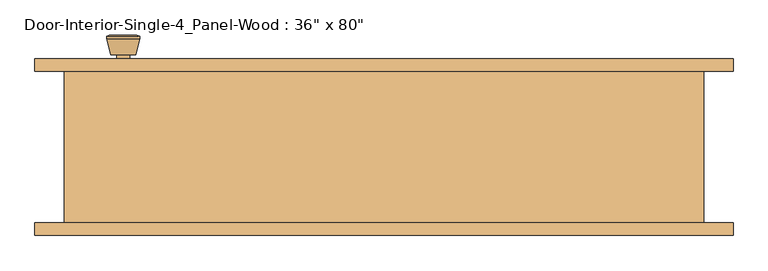
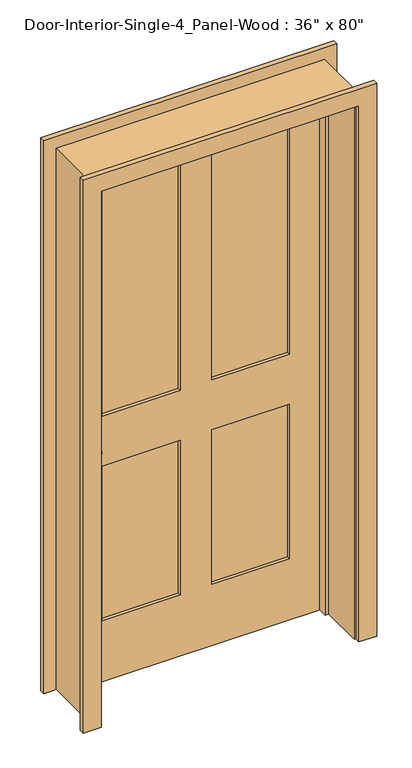
"""IFC4 building model written with IfcOpenShell, lengths in millimetres: door geometry."""

from ifc_helpers import new_model, si_unit, point, frame, frame_2d, origin, place, context, project, spatial, polyline, circle_curve, trimmed, segment, composite_curve, outline, extrude, faceted_brep, source, transform, mapped, element, save
from ifc_brep_helpers import plane_surface, cylinder_surface, revolved_surface, advanced_brep


def door_8a5afc22(model_context):
    return source(origin(), model_context, "Body", "SolidModel", [
        advanced_brep(
        [(-393.7, 70.2, 914.4), (-383.7, 70.2, 914.4), (-403.7, 70.2, 914.4), (-373.2241324, 21.2, 914.4), (-393.7, 21.2, 914.4), (-414.1758676, 21.2, 914.4), (-368.7, 23.0278681, 914.4), (-418.7, 23.0278681, 914.4), (-368.7, 26.4915463, 914.4), (-418.7, 26.4915463, 914.4), (-375.063764, 51.2, 914.4), (-412.336236, 51.2, 914.4), (-383.7, 51.2, 914.4), (-403.7, 51.2, 914.4)],
        [
            (0, 1),
            (1, 2, circle_curve(frame((-393.7, 70.2, 914.4), z_axis=(0.0, 1.0, 0.0), x_axis=(-1.0, 0.0, 0.0)), 10.0)),
            (2, 0),
            (2, 1, circle_curve(frame((-393.7, 70.2, 914.4), z_axis=(0.0, 1.0, 0.0), x_axis=(-1.0, 0.0, 0.0)), 10.0)),
            (3, 4),
            (4, 5),
            (5, 3, circle_curve(frame((-393.7, 21.2, 914.4), z_axis=(0.0, -1.0, 0.0), x_axis=(-1.0, 0.0, 0.0)), 20.4758676)),
            (3, 5, circle_curve(frame((-393.7, 21.2, 914.4), z_axis=(0.0, -1.0, 0.0), x_axis=(-1.0, 0.0, 0.0)), 20.4758676)),
            (6, 3),
            (5, 7),
            (7, 6, circle_curve(frame((-393.7, 23.0278681, 914.4), z_axis=(0.0, -1.0, 0.0), x_axis=(-1.0, 0.0, 0.0)), 25.0)),
            (6, 7, circle_curve(frame((-393.7, 23.0278681, 914.4), z_axis=(0.0, -1.0, 0.0), x_axis=(-1.0, 0.0, 0.0)), 25.0)),
            (8, 6),
            (7, 9),
            (9, 8, circle_curve(frame((-393.7, 26.4915463, 914.4), z_axis=(0.0, -1.0, 0.0), x_axis=(-1.0, 0.0, 0.0)), 25.0)),
            (8, 9, circle_curve(frame((-393.7, 26.4915463, 914.4), z_axis=(0.0, -1.0, 0.0), x_axis=(-1.0, 0.0, 0.0)), 25.0)),
            (10, 8),
            (9, 11),
            (11, 10, circle_curve(frame((-393.7, 51.2, 914.4), z_axis=(0.0, -1.0, 0.0), x_axis=(-1.0, 0.0, 0.0)), 18.636236)),
            (10, 11, circle_curve(frame((-393.7, 51.2, 914.4), z_axis=(0.0, -1.0, 0.0), x_axis=(-1.0, 0.0, 0.0)), 18.636236)),
            (12, 10),
            (11, 13),
            (13, 12, circle_curve(frame((-393.7, 51.2, 914.4), z_axis=(0.0, -1.0, 0.0), x_axis=(-1.0, 0.0, 0.0)), 10.0)),
            (12, 13, circle_curve(frame((-393.7, 51.2, 914.4), z_axis=(0.0, -1.0, 0.0), x_axis=(-1.0, 0.0, 0.0)), 10.0)),
            (1, 12),
            (13, 2),
        ],
        [
            plane_surface(frame((-393.7, 70.2, 914.4), z_axis=(0.0, 1.0, 0.0), x_axis=(-1.0, 0.0, 0.0))),
            plane_surface(frame((-393.7, 21.2, 914.4), z_axis=(0.0, -1.0, 0.0), x_axis=(-1.0, 0.0, 0.0))),
            revolved_surface(polyline([(-414.1758676, 21.2, 914.4), (-418.7, 23.0278681, 914.4)]), (-393.7, 70.2, 914.4), (0.0, 1.0, 0.0)),
            cylinder_surface(frame((-393.7, 70.2, 914.4), z_axis=(0.0, 1.0, 0.0), x_axis=(-1.0, 0.0, 0.0)), 25.0),
            revolved_surface(polyline([(-418.7, 26.4915463, 914.4), (-412.336236, 51.2, 914.4)]), (-393.7, 70.2, 914.4), (0.0, 1.0, 0.0)),
            plane_surface(frame((-393.7, 51.2, 914.4), z_axis=(0.0, 1.0, 0.0), x_axis=(-1.0, 0.0, 0.0))),
            cylinder_surface(frame((-393.7, 70.2, 914.4), z_axis=(0.0, 1.0, 0.0), x_axis=(-1.0, 0.0, 0.0)), 10.0),
        ],
        [
            (0, [[1, 2, 3]]),
            (0, [[-3, 4, -1]]),
            (1, [[5, 6, 7]]),
            (1, [[-6, -5, 8]]),
            (2, [[9, -7, 10, 11]]),
            (2, [[-10, -8, -9, 12]]),
            (3, [[13, -11, 14, 15]]),
            (3, [[-14, -12, -13, 16]]),
            (4, [[17, -15, 18, 19]]),
            (4, [[-18, -16, -17, 20]]),
            (5, [[21, -19, 22, 23]]),
            (5, [[-22, -20, -21, 24]]),
            (6, [[25, -23, 26, -2]]),
            (6, [[-26, -24, -25, -4]]),
        ],
    ),
        extrude(outline(composite_curve([segment(trimmed(circle_curve(frame_2d((914.4, -393.7)), 30.0), [point((914.4, -423.7))], [point((914.4, -363.7))], False, "CARTESIAN"), True, "CONTINUOUS"), segment(trimmed(circle_curve(frame_2d((914.4, -393.7)), 30.0), [point((914.4, -363.7))], [point((914.4, -423.7))], False, "CARTESIAN"), True, "CONTINUOUS")], self_intersect=False)), frame((0.0, 70.2, 0.0), z_axis=(0.0, 1.0, 0.0), x_axis=(0.0, 0.0, 1.0)), (0.0, 0.0, 1.0), 6.0),
        advanced_brep(
        [(-393.7, 117.125, 914.4), (-403.7, 117.125, 914.4), (-383.7, 117.125, 914.4), (-373.2241324, 166.125, 914.4), (-414.1758676, 166.125, 914.4), (-393.7, 166.125, 914.4), (-368.7, 164.2971319, 914.4), (-418.7, 164.2971319, 914.4), (-368.7, 160.8334537, 914.4), (-418.7, 160.8334537, 914.4), (-375.063764, 136.125, 914.4), (-412.336236, 136.125, 914.4), (-383.7, 136.125, 914.4), (-403.7, 136.125, 914.4)],
        [
            (0, 1),
            (1, 2, circle_curve(frame((-393.7, 117.125, 914.4), z_axis=(0.0, -1.0, 0.0), x_axis=(-1.0, 0.0, 0.0)), 10.0)),
            (2, 0),
            (2, 1, circle_curve(frame((-393.7, 117.125, 914.4), z_axis=(0.0, -1.0, 0.0), x_axis=(-1.0, 0.0, 0.0)), 10.0)),
            (3, 4, circle_curve(frame((-393.7, 166.125, 914.4), z_axis=(0.0, 1.0, 0.0), x_axis=(-1.0, 0.0, 0.0)), 20.4758676)),
            (4, 5),
            (5, 3),
            (4, 3, circle_curve(frame((-393.7, 166.125, 914.4), z_axis=(0.0, 1.0, 0.0), x_axis=(-1.0, 0.0, 0.0)), 20.4758676)),
            (6, 7, circle_curve(frame((-393.7, 164.2971319, 914.4), z_axis=(0.0, 1.0, 0.0), x_axis=(-1.0, 0.0, 0.0)), 25.0)),
            (7, 4),
            (3, 6),
            (7, 6, circle_curve(frame((-393.7, 164.2971319, 914.4), z_axis=(0.0, 1.0, 0.0), x_axis=(-1.0, 0.0, 0.0)), 25.0)),
            (8, 9, circle_curve(frame((-393.7, 160.8334537, 914.4), z_axis=(0.0, 1.0, 0.0), x_axis=(-1.0, 0.0, 0.0)), 25.0)),
            (9, 7),
            (6, 8),
            (9, 8, circle_curve(frame((-393.7, 160.8334537, 914.4), z_axis=(0.0, 1.0, 0.0), x_axis=(-1.0, 0.0, 0.0)), 25.0)),
            (10, 11, circle_curve(frame((-393.7, 136.125, 914.4), z_axis=(0.0, 1.0, 0.0), x_axis=(-1.0, 0.0, 0.0)), 18.636236)),
            (11, 9),
            (8, 10),
            (11, 10, circle_curve(frame((-393.7, 136.125, 914.4), z_axis=(0.0, 1.0, 0.0), x_axis=(-1.0, 0.0, 0.0)), 18.636236)),
            (12, 13, circle_curve(frame((-393.7, 136.125, 914.4), z_axis=(0.0, 1.0, 0.0), x_axis=(-1.0, 0.0, 0.0)), 10.0)),
            (13, 11),
            (10, 12),
            (13, 12, circle_curve(frame((-393.7, 136.125, 914.4), z_axis=(0.0, 1.0, 0.0), x_axis=(-1.0, 0.0, 0.0)), 10.0)),
            (1, 13),
            (12, 2),
        ],
        [
            plane_surface(frame((-393.7, 117.125, 914.4), z_axis=(0.0, -1.0, 0.0), x_axis=(-1.0, 0.0, 0.0))),
            plane_surface(frame((-393.7, 166.125, 914.4), z_axis=(0.0, 1.0, 0.0), x_axis=(-1.0, 0.0, 0.0))),
            revolved_surface(polyline([(-414.1758676, 166.125, 914.4), (-418.7, 164.2971319, 914.4)]), (-393.7, 117.125, 914.4), (0.0, -1.0, 0.0)),
            cylinder_surface(frame((-393.7, 117.125, 914.4), z_axis=(0.0, -1.0, 0.0), x_axis=(-1.0, 0.0, 0.0)), 25.0),
            revolved_surface(polyline([(-418.7, 160.8334537, 914.4), (-412.336236, 136.125, 914.4)]), (-393.7, 117.125, 914.4), (0.0, -1.0, 0.0)),
            plane_surface(frame((-393.7, 136.125, 914.4), z_axis=(0.0, -1.0, 0.0), x_axis=(-1.0, 0.0, 0.0))),
            cylinder_surface(frame((-393.7, 117.125, 914.4), z_axis=(0.0, -1.0, 0.0), x_axis=(-1.0, 0.0, 0.0)), 10.0),
        ],
        [
            (0, [[1, 2, 3]]),
            (0, [[-3, 4, -1]]),
            (1, [[5, 6, 7]]),
            (1, [[8, -7, -6]]),
            (2, [[9, 10, -5, 11]]),
            (2, [[12, -11, -8, -10]]),
            (3, [[13, 14, -9, 15]]),
            (3, [[16, -15, -12, -14]]),
            (4, [[17, 18, -13, 19]]),
            (4, [[20, -19, -16, -18]]),
            (5, [[21, 22, -17, 23]]),
            (5, [[24, -23, -20, -22]]),
            (6, [[-2, 25, -21, 26]]),
            (6, [[-4, -26, -24, -25]]),
        ],
    ),
        extrude(outline(composite_curve([segment(trimmed(circle_curve(frame_2d((914.4, -393.7)), 30.0), [point((914.4, -423.7))], [point((914.4, -363.7))], False, "CARTESIAN"), True, "CONTINUOUS"), segment(trimmed(circle_curve(frame_2d((914.4, -393.7)), 30.0), [point((914.4, -363.7))], [point((914.4, -423.7))], False, "CARTESIAN"), True, "CONTINUOUS")], self_intersect=False)), frame((0.0, 111.125, 0.0), z_axis=(0.0, 1.0, 0.0), x_axis=(0.0, 0.0, 1.0)), (0.0, 0.0, 1.0), 6.0),
        faceted_brep([(482.6, 111.125, 0.0), (482.6, -117.475, 0.0), (457.2, -117.475, 0.0), (457.2, 41.275, 0.0), (444.5, 41.275, 0.0), (444.5, 76.2, 0.0), (457.2, 76.2, 0.0), (457.2, 111.125, 0.0), (482.6, 111.125, 2057.4), (482.6, -117.475, 2057.4), (-482.6, -117.475, 2057.4), (-482.6, -117.475, 0.0), (-457.2, -117.475, 0.0), (-457.2, -117.475, 2032.0), (457.2, -117.475, 2032.0), (457.2, 41.275, 2032.0), (-457.2, 41.275, 2032.0), (-457.2, 41.275, 0.0), (-444.5, 41.275, 0.0), (-444.5, 41.275, 2019.3), (444.5, 41.275, 2019.3), (444.5, 76.2, 2019.3), (-444.5, 76.2, 2019.3), (-444.5, 76.2, 0.0), (-457.2, 76.2, 0.0), (-457.2, 76.2, 2032.0), (457.2, 76.2, 2032.0), (457.2, 111.125, 2032.0), (-457.2, 111.125, 2032.0), (-457.2, 111.125, 0.0), (-482.6, 111.125, 0.0), (-482.6, 111.125, 2057.4)], [[[0, 1, 2, 3, 4, 5, 6, 7]], [[1, 0, 8, 9]], [[2, 1, 9, 10, 11, 12, 13, 14]], [[3, 2, 14, 15]], [[4, 3, 15, 16, 17, 18, 19, 20]], [[5, 4, 20, 21]], [[6, 5, 21, 22, 23, 24, 25, 26]], [[7, 6, 26, 27]], [[0, 7, 27, 28, 29, 30, 31, 8]], [[9, 8, 31, 10]], [[15, 14, 13, 16]], [[21, 20, 19, 22]], [[27, 26, 25, 28]], [[30, 29, 24, 23, 18, 17, 12, 11]], [[10, 31, 30, 11]], [[16, 13, 12, 17]], [[22, 19, 18, 23]], [[28, 25, 24, 29]]]),
        extrude(outline(polyline([(2032.0, -457.2), (0.0, -457.2), (0.0, 457.2), (2032.0, 457.2), (2032.0, -457.2)]), holes=[polyline([(1912.9375, 57.15), (1912.9375, 336.55), (1009.65, 336.55), (1009.65, 57.15), (1912.9375, 57.15)]), polyline([(1009.65, -57.15), (1009.65, -336.55), (1912.9375, -336.55), (1912.9375, -57.15), (1009.65, -57.15)]), polyline([(819.15, 57.15), (819.15, 336.55), (231.775, 336.55), (231.775, 57.15), (819.15, 57.15)]), polyline([(231.775, -57.15), (231.775, -336.55), (819.15, -336.55), (819.15, -57.15), (231.775, -57.15)])]), frame((0.0, 76.2, 0.0), z_axis=(0.0, 1.0, 0.0), x_axis=(0.0, 0.0, 1.0)), (0.0, 0.0, 1.0), 34.925),
        extrude(outline(polyline([(336.55, 87.8416667), (57.15, 87.8416667), (57.15, 99.4833333), (336.55, 99.4833333), (336.55, 87.8416667)])), frame((0.0, 0.0, 1009.65), z_axis=(0.0, 0.0, 1.0), x_axis=(1.0, 0.0, 0.0)), (0.0, 0.0, 1.0), 903.2875),
        extrude(outline(polyline([(-57.15, 87.8416667), (-336.55, 87.8416667), (-336.55, 99.4833333), (-57.15, 99.4833333), (-57.15, 87.8416667)])), frame((0.0, 0.0, 1009.65), z_axis=(0.0, 0.0, 1.0), x_axis=(1.0, 0.0, 0.0)), (0.0, 0.0, 1.0), 903.2875),
        extrude(outline(polyline([(336.55, 87.8416667), (57.15, 87.8416667), (57.15, 99.4833333), (336.55, 99.4833333), (336.55, 87.8416667)])), frame((0.0, 0.0, 231.775), z_axis=(0.0, 0.0, 1.0), x_axis=(1.0, 0.0, 0.0)), (0.0, 0.0, 1.0), 587.375),
        extrude(outline(polyline([(-57.15, 87.8416667), (-336.55, 87.8416667), (-336.55, 99.4833333), (-57.15, 99.4833333), (-57.15, 87.8416667)])), frame((0.0, 0.0, 231.775), z_axis=(0.0, 0.0, 1.0), x_axis=(1.0, 0.0, 0.0)), (0.0, 0.0, 1.0), 587.375),
        extrude(outline(polyline([(0.0, 463.55), (0.0, 527.05), (2101.85, 527.05), (2101.85, -527.05), (0.0, -527.05), (0.0, -463.55), (2038.35, -463.55), (2038.35, 463.55), (0.0, 463.55)])), frame((0.0, 111.125, 0.0), z_axis=(0.0, 1.0, 0.0), x_axis=(0.0, 0.0, 1.0)), (0.0, 0.0, 1.0), 19.05),
        extrude(outline(polyline([(0.0, 463.55), (0.0, 527.05), (2101.85, 527.05), (2101.85, -527.05), (0.0, -527.05), (0.0, -463.55), (2038.35, -463.55), (2038.35, 463.55), (0.0, 463.55)])), frame((0.0, -136.525, 0.0), z_axis=(0.0, 1.0, 0.0), x_axis=(0.0, 0.0, 1.0)), (0.0, 0.0, 1.0), 19.05),
    ])


if __name__ == "__main__":
    model = new_model("IFC4")
    model_context = context("Model", 3, world=origin())
    ifc_project = project(units=[si_unit("LENGTHUNIT", "METRE", prefix="MILLI")], contexts=[model_context])
    site = spatial("IfcSite", under=ifc_project)
    building = spatial("IfcBuilding", under=site)
    placement = place(None, origin())
    door_shape = door_8a5afc22(model_context)
    element("IfcDoor", 1, ObjectType="Door-Interior-Single-4_Panel-Wood : 36\" x 80\"", at=placement, inside=building, context=model_context, shape_type="MappedRepresentation", body=[
        mapped(door_shape, transform((0.0, 0.0, 0.0), x_axis=(1.0, 0.0, 0.0), y_axis=(0.0, 1.0, 0.0), z_axis=(0.0, 0.0, 1.0))),
    ])
    save(model, "model.ifc")

# Revit data of these elements
# Type "Door-Interior-Single-4_Panel-Wood : 36\" x 80\""
#   Type Mark = "9"
#   Assembly Code = "C1020300"
#   Analytic Construction = "Wooden"
#   Top Rail = 0' - 4 11/16"
#   Thickness = 0' - 1 3/8"
#   Thermal Resistance (R) = 2.5876 (h·ft²·°F)/BTU
#   Swing Angle [instance default] = 90.00°
#   Stiles = 0' - 4 3/4"
#   Rough Width = 3' - 2"
#   Rough Height = 6' - 9"
#   Mullion = 0' - 4 1/2"
#   Lock Rail = 0' - 7 1/2"
#   Height = 6' - 8"
#   Width = 3' - 0"
#   Heat Transfer Coefficient (U) = 0.3865 BTU/(h·ft²·°F)
#   Bottom Rail = 0' - 9 1/8"
#   Trim Material = Cherry
#   Panel Material = Cherry
#   Frame Material = Cherry
#   Door Handle Material = Aluminum
#   Visual Light Transmittance = 0
#   Solar Heat Gain Coefficient = 0
#   Wall Closure = (empty or 0)
#   Function = (empty or 0)
# Element 1 (IfcDoor, "Door-Interior-Single-4_Panel-Wood : 36\" x 80\"")
#   Materials on its faces: "Cherry", "Aluminum"
# Materials
#   "Cherry": class "Wood", colour RGB 226 177 128, transparency 0, Description = "Prunus Serotina", Cost = 0
#   "Aluminum": class "Metal", colour RGB 247 247 247, transparency 0, Description = "Aluminum 6061", Cost = 0
